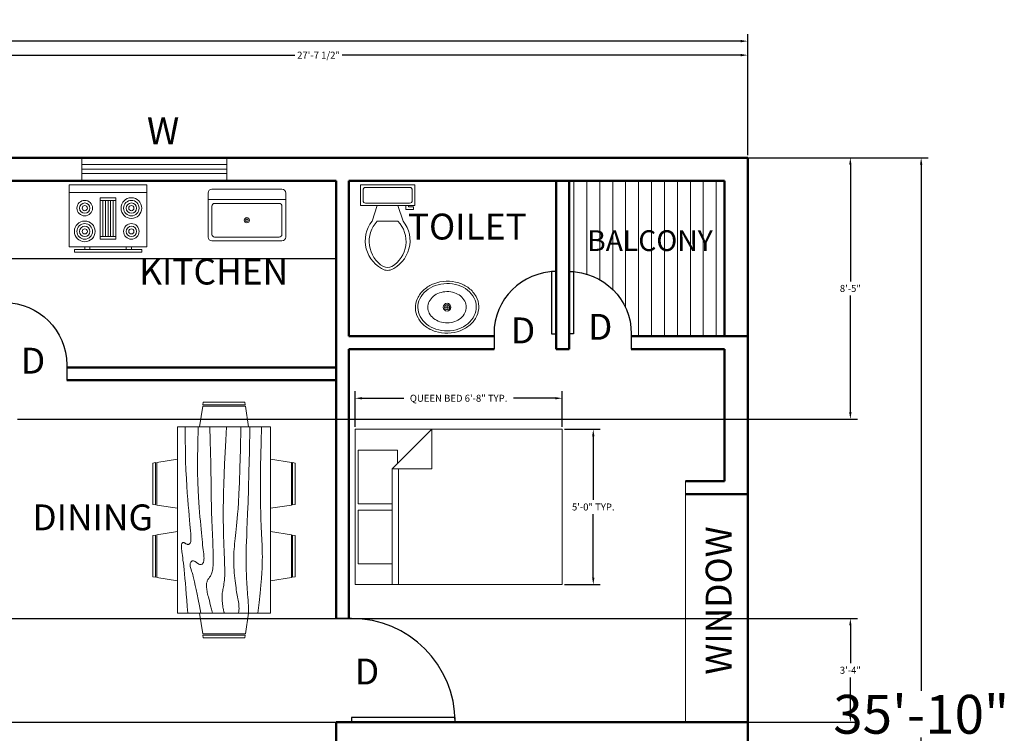
# Model space of a CAD drawing. Units: inches. Extents: x -15 to 796, y 111 to 651.
# Tile 6 of 6: x 416 to 796, y 376 to 651. Entities that reach past the tile are written whole.
import ezdxf

# ---------------------------------------------------------------- set-up
doc = ezdxf.new("R2010")
doc.units = ezdxf.units.IN
doc.header["$MEASUREMENT"] = 0
doc.layers.get('0').update_dxf_attribs({"color": 1})
for name, color, linetype, lineweight in [('A-ANNO-DIMS', 2, 'Continuous', 18), ('A-ANNO-TEXT', 7, 'Continuous', 18), ('A-AREA-IDEN', 7, 'Continuous', 25), ('A-DOOR', 3, 'Continuous', 25), ('A-EQPM', 8, 'Continuous', 20), ('A-FLOR-CASE', 8, 'Continuous', 25), ('A-FLOR-FIXT', 9, 'Continuous', 20), ('A-FLOR-PATT', 18, 'Continuous', 13), ('A-FURN', 8, 'Continuous', 18), ('A-GLAZ', 4, 'Continuous', 18), ('A-WALL', 7, 'Continuous', 50)]:
    doc.layers.add(name, color=color, linetype=linetype, lineweight=lineweight)
doc.styles.get("Standard").update_dxf_attribs({"font": 'arial.ttf'})
doc.dimstyles.get("Standard").update_dxf_attribs({"dimscale": 15, "dimtxt": 0.18, "dimasz": 0.18, "dimexe": 0.18, "dimexo": 0.0625, "dimgap": 0.09, "dimtad": 0, "dimtih": 1, "dimtoh": 1, "dimdec": 0, "dimzin": 0, "dimdsep": 46, "dimlunit": 3, "dimtxsty": 'Standard', "dimcen": 0.09, "dimadec": 0, "dimazin": 0, "dimtfac": 1, "dimtdec": 0, "dimtofl": 0, "dimtmove": 0, "dimatfit": 3, "dimfxl": 1, "dimtolj": 1, "dimtzin": 0, "dimarcsym": 0})

# ---------------------------------------------------------------- blocks, each defined once
blk = doc.blocks.new('Bed - Queen')
for p, q in [((0, -80.00003), (0, 0)), ((0, 0), (59.99999, 0)), ((59.99999, 0), (59.99999, -80.00003)), ((7.99999, -1.2), (28.79998, -1.2)), ((7.99999, -14.4), (7.99999, -1.2)), ((28.79998, -1.2), (28.79998, -14.4)), ((31.19999, -1.2), (51.99999, -1.2)), ((31.19999, -14.4), (31.19999, -1.2)), ((51.99999, -1.2), (51.99999, -16.4)), ((0, -14.4), (44.8, -14.4)), ((59.99999, -29.6), (44.8, -14.4)), ((44.8, -14.4), (44.8, -29.6)), ((44.8, -16.8), (0, -16.8)), ((51.99999, -16.4), (46.79936, -16.4)), ((44.8, -29.6), (59.99999, -29.6)), ((59.99999, -80.00003), (0, -80.00003))]:
    blk.add_line(p, q)
blk = doc.blocks.new('*U4')
for p, q in [((0, 0), (0, -6)), ((-40, 0), (-40, -6))]:
    blk.add_line(p, q)
blk.add_lwpolyline([(0, 0), (0, 40), (-1.75, 40), (-1.75, 0)], close=True)
blk.add_arc((0, 0), 40, 90, 180)
blk = doc.blocks.new('*U8')
for p, q in [((-24, 0), (-24, -6)), ((0, 0), (0, -6))]:
    blk.add_line(p, q)
blk.add_lwpolyline([(0, 0), (0, 24), (-1.75, 24), (-1.75, 0)], close=True)
blk.add_arc((0, 0), 24, 90, 180)
blk = doc.blocks.new('Sink - Oval top')
for p, q in [((-1, 0), (1, 0)), ((0, 1), (0, -1))]:
    blk.add_line(p, q)
for points in [[(-12.23, 0.39, 0.117634), (-11.46, -3.36, 0.104469), (-8.88, -6.8, 0.090016), (-5.08, -9.07, 0.08192), (-0.32, -10.02, 0.08192), (4.49, -9.38, 0.090016), (8.42, -7.36, 0.104469), (11.22, -4.09, 0.117634), (12.23, -0.39, 0.117634), (11.46, 3.36, 0.104469), (8.88, 6.8, 0.090016), (5.08, 9.07, 0.08192), (0.32, 10.02, 0.08192), (-4.49, 9.38, 0.090016), (-8.42, 7.36, 0.104469), (-11.22, 4.09, 0.117634)], [(-11.29, 0.16, 0.118622), (-10.52, -3.25, 0.104678), (-8.07, -6.36, 0.089562), (-4.54, -8.37, 0.081185), (-0.13, -9.15, 0.081185), (4.3, -8.49, 0.089562), (7.89, -6.58, 0.104678), (10.42, -3.55, 0.118622), (11.29, -0.16, 0.118622), (10.52, 3.25, 0.104678), (8.07, 6.36, 0.089562), (4.54, 8.37, 0.081185), (0.13, 9.15, 0.081185), (-4.3, 8.49, 0.089562), (-7.89, 6.58, 0.104678), (-10.42, 3.55, 0.118622)], [(-7.42, 0.08, 0.118283), (-6.91, -2.17, 0.104607), (-5.29, -4.21, 0.089718), (-2.97, -5.53, 0.081436), (-0.07, -6.04, 0.081436), (2.84, -5.59, 0.089718), (5.2, -4.33, 0.104607), (6.86, -2.32, 0.118283), (7.42, -0.08, 0.118283), (6.91, 2.17, 0.104607), (5.29, 4.21, 0.089718), (2.97, 5.53, 0.081436), (0.07, 6.04, 0.081436), (-2.84, 5.59, 0.089718), (-5.2, 4.33, 0.104607), (-6.86, 2.32, 0.118283)]]:
    blk.add_lwpolyline(points, format="xyb", close=True)
for radius in [1.5, 1]:
    blk.add_circle((0, 0), radius)
blk = doc.blocks.new('Toilet - top')
for p, q in [((9.5, -6), (9.5, -2)), ((-10, -8.5), (-8, -8.5)), ((-10, -9.5), (-10, -8.5)), ((-7, -9.5), (-10, -9.5)), ((-8, -8.5), (-8, -8)), ((-7, -8), (-7, -9.5)), ((-4, -8), (-6, -14)), ((4, -8), (6, -14)), ((4, -14), (-4, -14))]:
    blk.add_line(p, q)
blk.add_lwpolyline([(10.5, -8), (10.5, 0), (-10.5, 0), (-10.5, -8)], close=True)
for points in [[(-9.5, -2), (-9.5, -6)], [(8.5, -1), (-8.5, -1)], [(-8.5, -7), (8.5, -7)]]:
    blk.add_lwpolyline(points)
for centre, radius, start, end in [((-8.62, -1.88), 0.884, 81.8699, 188.1301), ((8.62, -1.88), 0.884, 351.8699, 98.1301), ((-8.62, -6.12), 0.884, 171.8699, 278.1301), ((8.62, -6.12), 0.884, 261.8699, 8.1301), ((3.52, -21.58), 12.17, 141.4691, 247.9714), ((4.2, -21.82), 11.33, 136.3677, 238.9468), ((-3.52, -21.58), 12.17, 292.0284, 38.5307), ((-4.2, -21.82), 11.33, 301.053, 43.6321), ((0, -27.88), 4, 245.7318, 294.2682), ((0, -29), 4, 254.8605, 285.1395)]:
    blk.add_arc(centre, radius, start, end)
blk = doc.blocks.new('Range-Oven - 30 in top')
for p, q in [((0, -3), (30, -3)), ((12, -6), (18, -6)), ((13, -20), (13, -6)), ((14, -6), (14, -20)), ((15, -20), (15, -6)), ((16, -6), (16, -20)), ((17, -20), (17, -6)), ((18, -20), (12, -20)), ((6, -24), (6, -25)), ((8, -25), (8, -24)), ((22, -25), (22, -24)), ((24, -24), (24, -25))]:
    blk.add_line(p, q)
for points in [[(0, -24), (0, 0), (30, 0), (30, -24)], [(12, -21), (12, -5), (18, -5), (18, -21)], [(2, -26), (2, -25), (28, -25), (28, -26)]]:
    blk.add_lwpolyline(points, close=True)
for centre, radius in [((6, -9), 4), ((6, -9), 3), ((6, -9), 2), ((24, -9), 3), ((24, -9), 2), ((6, -9), 1), ((24, -9), 1), ((6, -18), 3), ((24, -18), 4), ((24, -18), 3), ((6, -18), 2), ((6, -18), 1), ((24, -18), 2), ((24, -18), 1)]:
    blk.add_circle(centre, radius)
blk = doc.blocks.new('Sink-single - 30 in top')
blk.add_line((-15, -3.999996), (15, -3.999996))
for points in [[(-13.5, 0), (13.5, 0)], [(-15, -18.499996), (-15, -1.5)], [(15, -1.5), (15, -18.499996)], [(-13.5, -17.499996), (-13.5, -6.499996)], [(-12.5, -5.499996), (12.5, -5.499996)], [(13.5, -6.499996), (13.5, -17.499996)], [(12.5, -18.499996), (-12.5, -18.499996)], [(13.5, -19.999996), (-13.5, -19.999996)]]:
    blk.add_lwpolyline(points)
for radius in [1, 0.5]:
    blk.add_circle((0, -11.999996), radius)
for centre, radius, start, end in [((-13.5, -1.5), 1.5, 90, 180), ((13.5, -1.5), 1.5, 0, 90), ((-12.5, -6.499996), 1, 90, 180), ((12.5, -6.499996), 1, 0, 90), ((-13.5, -18.499996), 1.5, 180, 270), ((-12.5, -17.499996), 1, 180, 270), ((12.5, -17.499996), 1, 270, 0), ((13.5, -18.499996), 1.5, 270, 0)]:
    blk.add_arc(centre, radius, start, end)
blk = doc.blocks.new('*U13')
for p, q in [((-24, 0), (-24, -6)), ((0, 0), (0, -6))]:
    blk.add_line(p, q)
blk.add_lwpolyline([(0, 0), (0, 24), (-1.75, 24), (-1.75, 0)], close=True)
blk.add_arc((0, 0), 24, 90, 180)
blk = doc.blocks.new('Dining Set - 36 x 72 in.')
for p, q in [((-22, 27.5), (-22.1562, 26.50042)), ((-22, 27.5), (-6, 27.5)), ((-5.8437, 26.49966), (-6, 27.5)), ((6, 27.5), (5.8438, 26.50042)), ((6, 27.5), (22, 27.5)), ((22.1563, 26.49966), (22, 27.5)), ((-22.2343, 26.00059), (-23.4847, 17.99762)), ((-22.2304, 26), (-5.7608, 26)), ((-5.8416, 26.5), (-22.1534, 26.5)), ((-4.5152, 17.99762), (-5.7655, 25.99926)), ((5.7657, 26.00059), (4.5153, 17.99762)), ((5.7696, 26), (22.2392, 26)), ((22.1584, 26.5), (5.8466, 26.5)), ((23.4848, 17.99762), (22.2345, 25.99926)), ((36, 18), (-36, 18)), ((-36, 18), (-36, -18)), ((36, -18), (36, 18)), ((-45.5, 8), (-44.5004, 8.15617)), ((-45.5, 8), (-45.5, -8)), ((-44.5, -8.15843), (-44.5, 8.15338)), ((-44.0006, 8.23428), (-35.9976, 9.48474)), ((-44, 8.23041), (-44, -8.23915)), ((44.0006, 8.23428), (35.9976, 9.48474)), ((44, 8.23041), (44, -8.23915)), ((44.5, -8.15843), (44.5, 8.15338)), ((45.5, 8), (44.5005, 8.15617)), ((45.5, 8), (45.5, -8)), ((-44.4997, -8.15631), (-45.5, -8)), ((-35.9976, -9.48476), (-43.9993, -8.2345)), ((35.9976, -9.48476), (43.9993, -8.2345)), ((44.4997, -8.15631), (45.5, -8)), ((-36, -18), (36, -18)), ((-22.2343, -26.0006), (-23.4847, -17.99762)), ((-4.5152, -17.99762), (-5.7655, -25.99928)), ((5.7657, -26.0006), (4.5153, -17.99762)), ((23.4848, -17.99762), (22.2345, -25.99928)), ((-22.2304, -26), (-5.7608, -26)), ((-22, -27.5), (-22.1562, -26.50044)), ((-5.8416, -26.5), (-22.1534, -26.5)), ((-5.8437, -26.49967), (-6, -27.5)), ((5.7696, -26), (22.2392, -26)), ((6, -27.5), (5.8438, -26.50044)), ((22.1584, -26.5), (5.8466, -26.5)), ((22.1563, -26.49967), (22, -27.5)), ((-22, -27.5), (-6, -27.5)), ((6, -27.5), (22, -27.5))]:
    blk.add_line(p, q)
for points in [[(-36, 15), (-31.1772, 14.97754), (-26.8079, 14.91406), (-22.8538, 14.81543), (-19.276, 14.6875), (-16.0362, 14.53613), (-13.0957, 14.36718), (-10.4159, 14.18652), (-7.9583, 14), (-5.6904, 13.81315), (-3.6035, 13.63021), (-1.6954, 13.45508), (0.0365, 13.29166), (1.5945, 13.14388), (2.9811, 13.01562), (4.1988, 12.9108), (5.25, 12.83333), (6.1393, 12.78613), (6.8802, 12.76823), (7.4883, 12.77767), (7.9792, 12.8125), (8.3685, 12.87077), (8.6719, 12.95052), (8.9049, 13.0498), (9.0833, 13.16666), (9.2205, 13.29899), (9.3216, 13.44401), (9.3895, 13.59879), (9.4271, 13.76041), (9.4373, 13.92594), (9.4232, 14.09245), (9.3875, 14.257), (9.3333, 14.41666), (9.2638, 14.56917), (9.1836, 14.71484), (9.0975, 14.85465), (9.0104, 14.98958), (8.9272, 15.1206), (8.8529, 15.2487), (8.7922, 15.37483), (8.75, 15.5), (8.7305, 15.62467), (8.7344, 15.74739), (8.7617, 15.86621), (8.8125, 15.97916), (8.8867, 16.08431), (8.9844, 16.17968), (9.1055, 16.26334), (9.25, 16.33333), (9.4189, 16.38802), (9.6172, 16.42708), (9.8506, 16.45052), (10.125, 16.45833), (10.4463, 16.45052), (10.8203, 16.42708), (11.2529, 16.38802), (11.75, 16.33333), (12.3184, 16.26318), (12.9694, 16.17838), (13.7151, 16.07991), (14.5677, 15.96875), (15.5395, 15.84586), (16.6426, 15.71224), (17.8893, 15.56884), (19.2917, 15.41666), (20.859, 15.25667), (22.5879, 15.08984), (24.4721, 14.91715), (26.5052, 14.73958), (28.6809, 14.5581), (30.9929, 14.3737), (33.4347, 14.18733), (36, 14)], [(-36, 10), (-28.9766, 10.14274), (-23.1725, 10.20442), (-18.4241, 10.19775), (-14.5677, 10.13541), (-11.4399, 10.03011), (-8.877, 9.89453), (-6.7154, 9.74137), (-4.7917, 9.58333), (-2.9698, 9.43082), (-1.2246, 9.28515), (0.4415, 9.14534), (2.026, 9.01041), (3.5266, 8.87939), (4.9408, 8.7513), (6.266, 8.62516), (7.5, 8.5), (8.6411, 8.37549), (9.6914, 8.2539), (10.6538, 8.13818), (11.5312, 8.03125), (12.3267, 7.93603), (13.043, 7.85547), (13.6831, 7.79248), (14.25, 7.75), (14.7471, 7.7303), (15.1797, 7.73307), (15.5537, 7.75732), (15.875, 7.80208), (16.1494, 7.86637), (16.3828, 7.94922), (16.5811, 8.04964), (16.75, 8.16666), (16.8944, 8.29915), (17.0143, 8.44531), (17.1089, 8.60319), (17.1771, 8.77083), (17.218, 8.94629), (17.2305, 9.1276), (17.2137, 9.31282), (17.1667, 9.5), (17.0895, 9.6875), (16.987, 9.875), (16.8649, 10.0625), (16.7292, 10.25), (16.5856, 10.4375), (16.4401, 10.625), (16.2985, 10.8125), (16.1667, 11), (16.05, 11.18733), (15.9518, 11.3737), (15.8752, 11.5581), (15.8229, 11.73958), (15.798, 11.91715), (15.8034, 12.08984), (15.842, 12.25667), (15.9167, 12.41666), (16.0295, 12.56836), (16.1784, 12.70833), (16.3605, 12.83268), (16.5729, 12.9375), (16.8127, 13.01888), (17.0768, 13.07291), (17.3625, 13.0957), (17.6667, 13.08333), (17.9894, 13.03312), (18.3418, 12.94726), (18.7382, 12.82918), (19.1927, 12.68229), (19.7195, 12.51001), (20.3327, 12.31575), (21.0465, 12.10294), (21.875, 11.875), (22.8357, 11.63354), (23.959, 11.37304), (25.2786, 11.08618), (26.8282, 10.76562), (28.6414, 10.40405), (30.752, 9.99414), (33.1936, 9.52856), (36, 9)], [(-36, 5.5), (-30.7157, 5.3348), (-26.069, 5.20963), (-21.9946, 5.11767), (-18.4271, 5.05208), (-15.3009, 5.00602), (-12.5508, 4.97265), (-10.1112, 4.94515), (-7.9167, 4.91666), (-5.909, 4.88167), (-4.0586, 4.83984), (-2.3429, 4.79215), (-0.7396, 4.73958), (0.7739, 4.6831), (2.22, 4.6237), (3.6213, 4.56233), (5, 4.5), (6.373, 4.43782), (7.7344, 4.3776), (9.0723, 4.32129), (10.375, 4.27083), (11.6309, 4.22819), (12.8281, 4.19531), (13.9551, 4.17415), (15, 4.16666), (15.954, 4.17448), (16.819, 4.19791), (17.6001, 4.23698), (18.3021, 4.29166), (18.9299, 4.36198), (19.4883, 4.44791), (19.9823, 4.54948), (20.4167, 4.66666), (20.7969, 4.79899), (21.1302, 4.94401), (21.4245, 5.09879), (21.6875, 5.26041), (21.9271, 5.42594), (22.1511, 5.59245), (22.3672, 5.757), (22.5834, 5.91666), (22.8065, 6.06868), (23.0404, 6.21093), (23.2879, 6.34147), (23.5521, 6.45833), (23.8358, 6.55957), (24.142, 6.64323), (24.4735, 6.70735), (24.8334, 6.75), (25.2235, 6.76969), (25.642, 6.76692), (26.0858, 6.74267), (26.5521, 6.69791), (27.0379, 6.63362), (27.5404, 6.55078), (28.0565, 6.45036), (28.5834, 6.33333), (29.1242, 6.19987), (29.7071, 6.04687), (30.3661, 5.87044), (31.1354, 5.66666), (32.0493, 5.43164), (33.142, 5.16146), (34.4475, 4.85221), (36, 4.5)], [(-36, -1), (-30.7915, -0.6591), (-26.0195, -0.38216), (-21.6519, -0.16284), (-17.6563, 0.00521), (-14.0005, 0.12833), (-10.6523, 0.21289), (-7.5796, 0.26522), (-4.75, 0.29166), (-2.134, 0.29793), (0.2878, 0.28711), (2.5317, 0.26163), (4.6146, 0.22396), (6.5529, 0.17651), (8.3633, 0.12174), (10.0623, 0.06209), (11.6667, 0), (13.1899, -0.06201), (14.6341, -0.1211), (15.9982, -0.17432), (17.2813, -0.21875), (18.4823, -0.25147), (19.6003, -0.26953), (20.6343, -0.27002), (21.5834, -0.25), (22.4481, -0.20768), (23.2357, -0.14584), (23.9549, -0.06836), (24.6146, 0.02083), (25.2235, 0.11784), (25.7904, 0.21875), (26.3241, 0.31966), (26.8334, 0.41666), (27.3265, 0.50618), (27.8099, 0.58593), (28.2894, 0.65397), (28.7709, 0.70833), (29.2601, 0.74707), (29.763, 0.76823), (30.2855, 0.76985), (30.8334, 0.75), (31.4088, 0.70784), (31.9994, 0.64713), (32.589, 0.57275), (33.1615, 0.48958), (33.7008, 0.4025), (34.1908, 0.3164), (34.6153, 0.23616), (34.9584, 0.16666), (35.2099, 0.11165), (35.3848, 0.07031), (35.504, 0.04069), (35.5886, 0.02083), (35.6594, 0.00879), (35.7377, 0.0026), (35.8442, 0.00032), (36, 0)], [(-36, -6.5), (-27.1843, -6.31267), (-20.084, -6.1263), (-14.469, -5.9419), (-10.1094, -5.76042), (-6.7752, -5.58285), (-4.2363, -5.41016), (-2.2629, -5.24333), (-0.625, -5.08334), (0.8708, -4.93099), (2.2715, -4.78646), (3.5872, -4.64974), (4.8281, -4.52084), (6.0046, -4.39974), (7.127, -4.28646), (8.2053, -4.18099), (9.25, -4.08334), (10.2705, -3.99382), (11.2734, -3.91407), (12.2647, -3.84603), (13.25, -3.79167), (14.2354, -3.75293), (15.2266, -3.73177), (16.2295, -3.73015), (17.25, -3.75), (18.2912, -3.79248), (19.3451, -3.85547), (20.4009, -3.93604), (21.4479, -4.03125), (22.4754, -4.13819), (23.4727, -4.25391), (24.4289, -4.37549), (25.3334, -4.5), (26.1785, -4.62492), (26.9694, -4.74935), (27.7145, -4.87281), (28.4219, -4.99479), (29.1, -5.11483), (29.7572, -5.23242), (30.4016, -5.34709), (31.0417, -5.45834), (31.6837, -5.56437), (32.3262, -5.65821), (32.9658, -5.73153), (33.599, -5.77604), (34.2224, -5.78345), (34.8327, -5.74545), (35.4264, -5.65373), (36, -5.5)], [(-36, -10), (-26.4022, -9.81299), (-18.4675, -9.62891), (-11.9839, -9.45069), (-6.7396, -9.28125), (-2.5226, -9.12354), (0.8789, -8.98047), (3.6769, -8.85498), (6.0833, -8.75), (8.2767, -8.66765), (10.3021, -8.60677), (12.1712, -8.56543), (13.8958, -8.54167), (15.4876, -8.53353), (16.9583, -8.53907), (18.3197, -8.55632), (19.5834, -8.58334), (20.7616, -8.61841), (21.8685, -8.66081), (22.9188, -8.71004), (23.9271, -8.76563), (24.9081, -8.82707), (25.8763, -8.89388), (26.8465, -8.96558), (27.8334, -9.04167), (28.8474, -9.12118), (29.8828, -9.20117), (30.93, -9.27824), (31.9792, -9.34896), (33.0205, -9.40991), (34.0443, -9.45768), (35.0407, -9.48885), (36, -9.5)], [(-36, -14.5), (-30.0881, -14.33513), (-25.0332, -14.21224), (-20.7312, -14.12647), (-17.0781, -14.07292), (-13.97, -14.04671), (-11.3027, -14.04297), (-8.9724, -14.05681), (-6.875, -14.08334), (-4.9224, -14.11833), (-3.0905, -14.16016), (-1.3709, -14.20785), (0.2448, -14.26042), (1.7647, -14.3169), (3.1973, -14.3763), (4.5507, -14.43767), (5.8333, -14.5), (7.0554, -14.5621), (8.235, -14.62175), (9.3922, -14.67652), (10.5469, -14.72396), (11.7192, -14.76164), (12.929, -14.78711), (14.1965, -14.79794), (15.5417, -14.79167), (16.9933, -14.76424), (18.6152, -14.70508), (20.4804, -14.60197), (22.6615, -14.44271), (25.2312, -14.21509), (28.2624, -13.9069), (31.8277, -13.50594), (36, -13)]]:
    blk.add_lwpolyline(points)
blk = doc.blocks.new('*D16')
at = {"layer": 'A-ANNO-DIMS', "color": 0, "lineweight": -2, "transparency": 16777216}
for p, q in [((30.18, 599.06), (30.18, 645.85)), ((32.88, 643.15), (336.57, 643.15)), ((694.48, 643.15), (390.8, 643.15)), ((697.18, 599.06), (697.18, 645.85))]:
    blk.add_line(p, q, dxfattribs=at)
at = {"layer": 'A-ANNO-DIMS', "color": 0, "transparency": 16777216}
for points in [[(32.88, 643.6), (32.88, 642.7), (30.18, 643.15)], [(694.48, 643.6), (694.48, 642.7), (697.18, 643.15)]]:
    blk.add_solid(points, dxfattribs=at)
at = {"layer": 'Defpoints', "color": 0, "transparency": 16777216}
for p in [(697.18, 643.15), (30.18, 598.13), (697.18, 598.13)]:
    blk.add_point(p, dxfattribs=at)
at = {"layer": 'A-ANNO-DIMS', "color": 0, "transparency": 16777216, "insert": (363.68, 643.15), "char_height": 2.7, "attachment_point": 5}
blk.add_mtext('\\A1;{\\H5.55556x;55\'-7"}', dxfattribs=at)
blk = doc.blocks.new('*D17')
at = {"layer": 'A-ANNO-DIMS', "color": 0, "lineweight": -2, "transparency": 16777216}
for p, q in [((698.12, 598.13), (766.83, 598.13)), ((764.13, 595.43), (764.13, 392.14)), ((764.13, 170.83), (764.13, 374.11)), ((698.12, 168.13), (766.83, 168.13))]:
    blk.add_line(p, q, dxfattribs=at)
at = {"layer": 'A-ANNO-DIMS', "color": 0, "transparency": 16777216}
for points in [[(763.68, 595.43), (764.58, 595.43), (764.13, 598.13)], [(763.68, 170.83), (764.58, 170.83), (764.13, 168.13)]]:
    blk.add_solid(points, dxfattribs=at)
at = {"layer": 'Defpoints', "color": 0, "transparency": 16777216}
for p in [(697.18, 598.13), (697.18, 168.13), (764.13, 168.13)]:
    blk.add_point(p, dxfattribs=at)
at = {"layer": 'A-ANNO-DIMS', "color": 0, "transparency": 16777216, "insert": (764.13, 383.13), "char_height": 2.7, "attachment_point": 5}
blk.add_mtext('\\A1;{\\H5.55556x;35\'-10"}', dxfattribs=at)
blk = doc.blocks.new('WIN-KITCHEN-56IN')
for p, q in [((0, 6.34), (56, 6.34)), ((0, 4.5), (56, 4.5)), ((0, 2.84), (56, 2.84))]:
    blk.add_line(p, q)
blk.add_lwpolyline([(0, 9), (56, 9), (56, 0), (0, 0)], close=True)
blk = doc.blocks.new('*D39')
at = {"layer": 'A-ANNO-DIMS', "color": 0, "lineweight": -2, "transparency": 16777216}
for p, q in [((545.51, 494.14), (545.51, 507.9)), ((625.51, 494.14), (625.51, 507.9)), ((548.21, 505.2), (564.31, 505.2)), ((622.81, 505.2), (606.72, 505.2))]:
    blk.add_line(p, q, dxfattribs=at)
at = {"layer": 'A-ANNO-DIMS', "color": 0, "transparency": 16777216}
for points in [[(548.21, 505.65), (548.21, 504.75), (545.51, 505.2)], [(622.81, 505.65), (622.81, 504.75), (625.51, 505.2)]]:
    blk.add_solid(points, dxfattribs=at)
at = {"layer": 'Defpoints', "color": 0, "transparency": 16777216}
for p in [(545.51, 505.2), (545.51, 493.2), (625.51, 493.2)]:
    blk.add_point(p, dxfattribs=at)
at = {"layer": 'A-ANNO-DIMS', "color": 0, "transparency": 16777216, "insert": (585.51, 505.2), "char_height": 2.7, "attachment_point": 5}
blk.add_mtext('\\A1;QUEEN BED 6\'-8" TYP.', dxfattribs=at)
blk = doc.blocks.new('*D40')
at = {"layer": 'A-ANNO-DIMS', "color": 0, "lineweight": -2, "transparency": 16777216}
for p, q in [((626.45, 493.2), (640.21, 493.2)), ((637.51, 490.5), (637.51, 465.93)), ((637.51, 435.9), (637.51, 460.48)), ((626.45, 433.2), (640.21, 433.2))]:
    blk.add_line(p, q, dxfattribs=at)
at = {"layer": 'A-ANNO-DIMS', "color": 0, "transparency": 16777216}
for points in [[(637.06, 490.5), (637.96, 490.5), (637.51, 493.2)], [(637.06, 435.9), (637.96, 435.9), (637.51, 433.2)]]:
    blk.add_solid(points, dxfattribs=at)
at = {"layer": 'Defpoints', "color": 0, "transparency": 16777216}
for p in [(625.51, 493.2), (637.51, 493.2), (625.51, 433.2)]:
    blk.add_point(p, dxfattribs=at)
at = {"layer": 'A-ANNO-DIMS', "color": 0, "transparency": 16777216, "insert": (637.51, 463.2), "char_height": 2.7, "attachment_point": 5}
blk.add_mtext('\\A1;5\'-0" TYP.', dxfattribs=at)
blk = doc.blocks.new('*D75')
at = {"layer": 'A-ANNO-DIMS', "color": 0, "lineweight": -2, "transparency": 16777216}
for p, q in [((415.12, 598.13), (739.48, 598.13)), ((736.78, 595.43), (736.78, 550.36)), ((736.78, 499.83), (736.78, 544.9)), ((415.12, 497.13), (739.48, 497.13))]:
    blk.add_line(p, q, dxfattribs=at)
at = {"layer": 'A-ANNO-DIMS', "color": 0, "transparency": 16777216}
for points in [[(736.33, 595.43), (737.23, 595.43), (736.78, 598.13)], [(736.33, 499.83), (737.23, 499.83), (736.78, 497.13)]]:
    blk.add_solid(points, dxfattribs=at)
at = {"layer": 'Defpoints', "color": 0, "transparency": 16777216}
for p in [(414.18, 598.13), (414.18, 497.13), (736.78, 497.13)]:
    blk.add_point(p, dxfattribs=at)
at = {"layer": 'A-ANNO-DIMS', "color": 0, "transparency": 16777216, "insert": (736.78, 547.63), "char_height": 2.7, "attachment_point": 5}
blk.add_mtext('\\A1;8\'-5"', dxfattribs=at)
blk = doc.blocks.new('*D78')
at = {"layer": 'A-ANNO-DIMS', "color": 0, "lineweight": -2, "transparency": 16777216}
for p, q in [((185.12, 420.13), (739.48, 420.13)), ((736.78, 417.43), (736.78, 402.86)), ((736.78, 382.83), (736.78, 397.4)), ((185.87, 380.13), (739.48, 380.13))]:
    blk.add_line(p, q, dxfattribs=at)
at = {"layer": 'A-ANNO-DIMS', "color": 0, "transparency": 16777216}
for points in [[(736.33, 417.43), (737.23, 417.43), (736.78, 420.13)], [(736.33, 382.83), (737.23, 382.83), (736.78, 380.13)]]:
    blk.add_solid(points, dxfattribs=at)
at = {"layer": 'Defpoints', "color": 0, "transparency": 16777216}
for p in [(184.18, 420.13), (736.78, 420.13), (184.93, 380.13)]:
    blk.add_point(p, dxfattribs=at)
at = {"layer": 'A-ANNO-DIMS', "color": 0, "transparency": 16777216, "insert": (736.78, 400.13), "char_height": 2.7, "attachment_point": 5}
blk.add_mtext('\\A1;3\'-4"', dxfattribs=at)
blk = doc.blocks.new('*D83')
at = {"layer": 'A-ANNO-DIMS', "color": 0, "lineweight": -2, "transparency": 16777216}
for p, q in [((365.68, 583.73), (365.68, 640.43)), ((697.18, 599.06), (697.18, 640.43)), ((368.38, 637.73), (522.28, 637.73)), ((694.48, 637.73), (540.59, 637.73))]:
    blk.add_line(p, q, dxfattribs=at)
at = {"layer": 'A-ANNO-DIMS', "color": 0, "transparency": 16777216}
for points in [[(368.38, 638.18), (368.38, 637.28), (365.68, 637.73)], [(694.48, 638.18), (694.48, 637.28), (697.18, 637.73)]]:
    blk.add_solid(points, dxfattribs=at)
at = {"layer": 'Defpoints', "color": 0, "transparency": 16777216}
for p in [(697.18, 637.73), (697.18, 598.13), (365.68, 582.8)]:
    blk.add_point(p, dxfattribs=at)
at = {"layer": 'A-ANNO-DIMS', "color": 0, "transparency": 16777216, "insert": (531.43, 637.73), "char_height": 2.7, "attachment_point": 5}
blk.add_mtext('\\A1;27\'-7 1/2"', dxfattribs=at)

msp = doc.modelspace()

# ---------------------------------------------------------------- hatches: boundary and pattern name
at = {"layer": 'A-FLOR-PATT'}
h = msp.add_hatch(dxfattribs=at)
h.set_pattern_fill('_USER', color=256, scale=5, angle=90, pattern_type=0)
h.set_pattern_definition([(90, (0, 0), (-5, 3e-16), [])])
h.paths.add_polyline_path([(99.18, 589.13), (39.18, 589.13), (39.18, 529.13), (75.18, 529.13), (75.18, 530.13, -0.392996), (97.43, 554.06), (97.43, 554.13), (99.18, 554.13)])
h.paths.add_polyline_path([(688.18, 589.13), (628.18, 589.13), (628.18, 554.13), (629.93, 554.13), (629.93, 554.06, -0.392996), (652.18, 530.13), (652.18, 529.13), (688.18, 529.13)])
h.paths.add_polyline_path([(40.9, 557.57), (98.32, 557.57), (98.32, 574.06), (40.9, 574.06)], flags=24)
h.paths.add_polyline_path([(628.32, 557.57), (685.73, 557.57), (685.73, 574.06), (628.32, 574.06)], flags=24)

# ---------------------------------------------------------------- linework, layer by layer
at = {"layer": 'A-FLOR-CASE'}
msp.add_line((410.18, 559.13), (538.18, 559.13), dxfattribs=at)
at = {"layer": 'A-GLAZ'}
msp.add_line((673.18, 473.13), (673.18, 380.13), dxfattribs=at)
at = {"layer": 'A-WALL'}
for p, q in [((405.18, 598.13), (697.18, 598.13)), ((697.18, 598.13), (697.18, 468.13)), ((410.18, 589.13), (538.18, 589.13)), ((538.18, 589.13), (538.18, 420.13)), ((543.18, 529.13), (543.18, 589.13)), ((543.18, 589.13), (688.18, 589.13)), ((623.18, 589.13), (623.18, 524.13)), ((628.18, 589.13), (628.18, 524.13)), ((688.18, 589.13), (688.18, 529.13)), ((543.18, 529.13), (599.18, 529.13)), ((652.18, 529.13), (688.18, 529.13)), ((688.18, 529.13), (697.18, 529.13)), ((543.18, 420.13), (543.18, 524.13)), ((543.18, 524.13), (599.18, 524.13)), ((623.18, 524.13), (628.18, 524.13)), ((652.18, 524.13), (688.18, 524.13)), ((688.18, 524.13), (688.18, 473.13)), ((434.18, 517.13), (538.18, 517.13)), ((434.18, 512.13), (538.18, 512.13)), ((673.18, 473.13), (688.18, 473.13)), ((673.18, 468.13), (697.18, 468.13)), ((697.18, 468.13), (697.18, 380.13)), ((538.18, 380.13), (697.18, 380.13)), ((538.18, 380.13), (538.18, 371.13)), ((697.18, 380.13), (697.18, 227.13))]:
    msp.add_line(p, q, dxfattribs=at)

# ---------------------------------------------------------------- block references
at = {"layer": 'A-DOOR'}
msp.add_blockref('*U8', (623.18, 530.13), dxfattribs=at)
at = {"layer": 'A-DOOR', "xscale": -1}
for name, p in [('*U8', (628.18, 530.13)), ('*U13', (410.18, 518.13))]:
    msp.add_blockref(name, p, dxfattribs=at)
at = {"layer": 'A-DOOR', "rotation": 270}
msp.add_blockref('*U4', (544.18, 380.13), dxfattribs=at)
at = {"layer": 'A-EQPM', "xscale": -1}
msp.add_blockref('Range-Oven - 30 in top', (465.15, 587.65), dxfattribs=at)
at = {"layer": 'A-FLOR-FIXT', "xscale": -1}
for name, p in [('Sink-single - 30 in top', (503.77, 585.96)), ('Toilet - top', (558.1, 587.6)), ('Sink - Oval top', (581.06, 540.37))]:
    msp.add_blockref(name, p, dxfattribs=at)
at = {"layer": 'A-FURN', "xscale": -1, "rotation": 90}
msp.add_blockref('Dining Set - 36 x 72 in.', (494.93, 458.19), dxfattribs=at)
at = {"layer": 'A-FURN', "rotation": 90.00000000000003}
msp.add_blockref('Bed - Queen', (545.51, 433.2), dxfattribs=at)
at = {"layer": 'A-GLAZ', "extrusion": (0, 0, -1), "zscale": -1}
msp.add_blockref('WIN-KITCHEN-56IN', (-496, 589.13), dxfattribs=at)

# ---------------------------------------------------------------- texts
at = {"layer": 'A-ANNO-TEXT'}
msp.add_text('WINDOW', height=10, rotation=90, dxfattribs=at).set_placement((690.91, 398.41))
at = {"layer": 'A-ANNO-TEXT', "attachment_point": 3}
for s, width, gutter_width, insert, char_height in [('W', 19.9719, 52.27, (477.66, 613.77), 10.45), ('D', 13.2435, 1, (615.1, 536.41), 10), ('D', 13.2435, 1, (644.87, 537.79), 10), ('D', 13.2435, 1, (425.88, 524.71), 10), ('D', 13.2435, 1, (554.85, 404.64), 10)]:
    msp.add_mtext_dynamic_manual_height_columns(s, width=width, gutter_width=gutter_width, heights=[0], dxfattribs=dict(at, insert=insert, char_height=char_height))
at = {"layer": 'A-AREA-IDEN', "attachment_point": 3}
for s, width, insert, char_height in [('TOILET', 20.6028, (611.83, 576.52), 10), ('BALCONY', 13.9372, (683.64, 570.08), 8), ('KITCHEN', 30.3121, (519.67, 559.13), 10), ('DINING', 31.9005, (467.43, 464.19), 10)]:
    msp.add_mtext_dynamic_manual_height_columns(s, width=width, gutter_width=50, heights=[0], dxfattribs=dict(at, insert=insert, char_height=char_height))

# ---------------------------------------------------------------- dimensions: what is measured, and where the dimension line sits
at = {"layer": 'A-ANNO-DIMS'}
dim = msp.add_linear_dim(base=(697.18, 643.15), p1=(30.18, 598.13), p2=(697.18, 598.13), text='{\\H5.55556x;<>}', dimstyle='Standard', override={"dimclrd": 0, "dimclre": 0, "dimclrt": 0}, dxfattribs=at)
dim.commit()
dim.dimension.update_dxf_attribs({"geometry": '*D16', "text_midpoint": (363.68, 643.15), "dimtype": 160})
dim = msp.add_linear_dim(base=(697.18, 637.73), p1=(365.68, 582.8), p2=(697.18, 598.13), dimstyle='Standard', override={"dimdec": 1, "dimlfac": 1, "dimrnd": 0, "dimzin": 1, "dimdsep": 46, "dimlunit": 4, "dimfrac": 2}, dxfattribs=at)
dim.commit()
dim.dimension.update_dxf_attribs({"geometry": '*D83', "text_midpoint": (531.43, 637.73)})
for base, p1, p2, picture, middle in [((736.78, 497.13), (414.18, 598.13), (414.18, 497.13), '*D75', (736.78, 547.63)), ((736.78, 420.13), (184.93, 380.13), (184.18, 420.13), '*D78', (736.78, 400.13))]:
    dim = msp.add_linear_dim(base=base, p1=p1, p2=p2, angle=90, dimstyle='Standard', override={"dimdec": 1, "dimlfac": 1, "dimrnd": 0, "dimzin": 1, "dimdsep": 46, "dimlunit": 4, "dimfrac": 2}, dxfattribs=at)
    dim.commit()
    dim.dimension.update_dxf_attribs({"geometry": picture, "text_midpoint": middle})
for base, p1, p2, angle, text, override, picture, middle in [((764.13, 168.13), (697.18, 598.13), (697.18, 168.13), 90, '{\\H5.55556x;<>}', {"dimclrd": 0, "dimclre": 0, "dimclrt": 0}, '*D17', (764.13, 383.13)), ((545.51, 505.2), (625.51, 493.2), (545.51, 493.2), 180, 'QUEEN BED <> TYP.', {"dimdec": 1, "dimlfac": 1, "dimrnd": 0, "dimzin": 1, "dimdsep": 46, "dimlunit": 4, "dimfrac": 2}, '*D39', (585.51, 505.2)), ((637.51, 493.2), (625.51, 433.2), (625.51, 493.2), 90, '<> TYP.', {"dimdec": 1, "dimlfac": 1, "dimrnd": 0, "dimzin": 1, "dimdsep": 46, "dimlunit": 4, "dimfrac": 2}, '*D40', (637.51, 463.2))]:
    dim = msp.add_linear_dim(base=base, p1=p1, p2=p2, angle=angle, text=text, dimstyle='Standard', override=override, dxfattribs=at)
    dim.commit()
    dim.dimension.update_dxf_attribs({"geometry": picture, "text_midpoint": middle})

doc.saveas('drawing.dxf')
